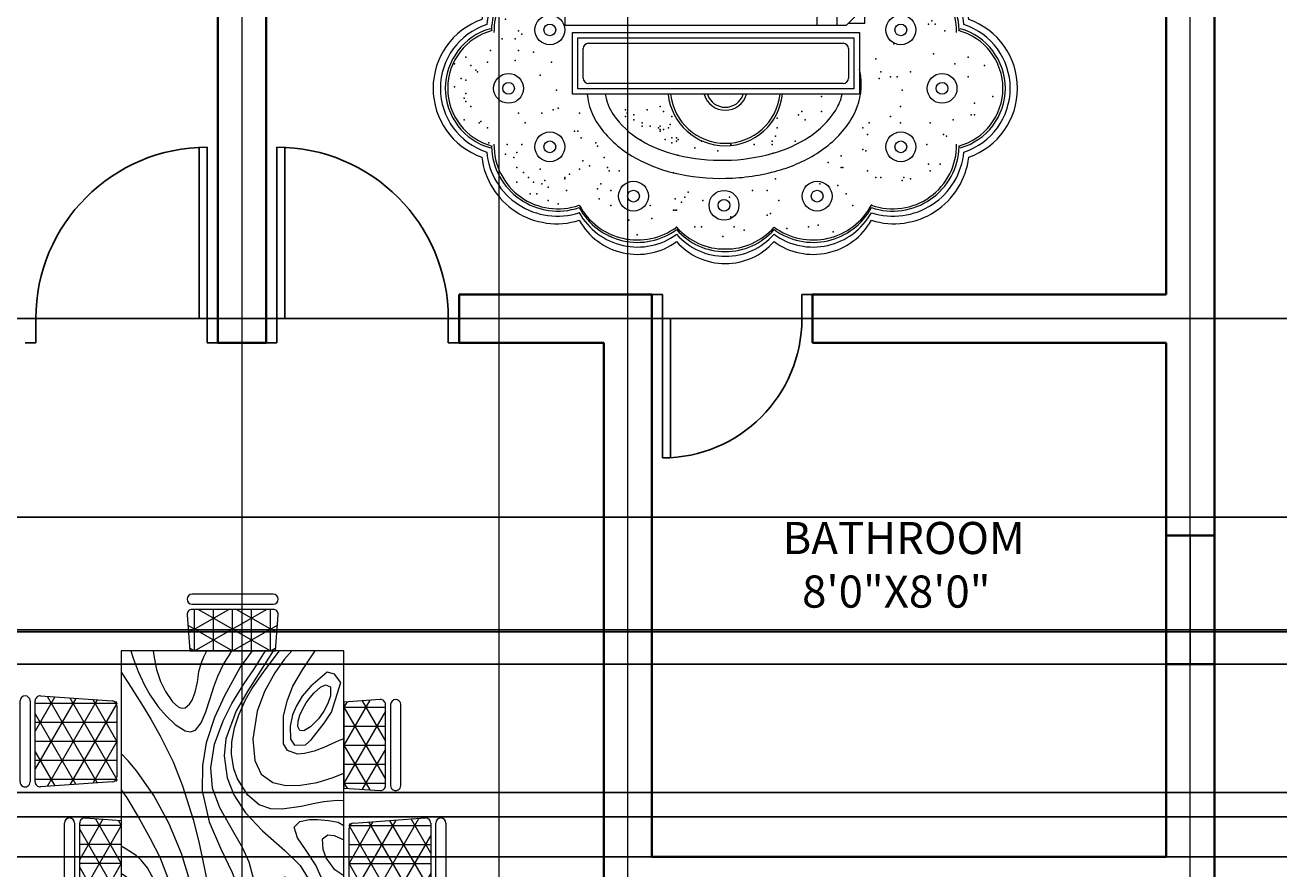
# Model space of a CAD drawing. Units: inches. Extents: x 5716 to 6907, y 12769 to 13594.
# Tile 15 of 17: x 6414 to 6648, y 13192 to 13349. Entities that reach past the tile are written whole.
import ezdxf

# ---------------------------------------------------------------- set-up
doc = ezdxf.new("R2010")
doc.units = ezdxf.units.IN
doc.linetypes.add('ACAD_ISO03W100', pattern=[30, 12, -18])
for name, color, linetype, lineweight in [('A-ANNO-DIMS', 2, 'Continuous', 18), ('A-AREA-IDEN', 7, 'Continuous', 18), ('A-DOOR', 4, 'Continuous', 25), ('A-FLOR-OVHD', 8, 'ACAD_ISO03W100', 18), ('A-FURN', 8, 'Continuous', 18), ('A-GLAZ', 4, 'Continuous', 18), ('A-GRID', 8, 'Continuous', 13), ('A-WALL', 7, 'Continuous', 35)]:
    doc.layers.add(name, color=color, linetype=linetype, lineweight=lineweight)
doc.styles.get("Standard").update_dxf_attribs({"font": 'arial.ttf'})
doc.dimstyles.get("Standard").update_dxf_attribs({"dimtxt": 0.18, "dimasz": 0.18, "dimexe": 0.18, "dimexo": 0.0625, "dimgap": 0.09, "dimtad": 0, "dimtih": 1, "dimtoh": 1, "dimdec": 4, "dimzin": 0, "dimdsep": 46, "dimtxsty": 'Standard', "dimcen": 0.09, "dimadec": 0, "dimazin": 0, "dimtfac": 1, "dimtdec": 4, "dimtofl": 0, "dimtmove": 0, "dimatfit": 3, "dimfxl": 1, "dimtolj": 1, "dimtzin": 0, "dimarcsym": 0})

# ---------------------------------------------------------------- blocks, each defined once
blk = doc.blocks.new('A$C1EC128A1')
for p, q in [((0.1147, 3.56), (3.0187, 3.56)), ((0.1147, 3.555), (0.1147, 3.511)), ((3.0187, 3.555), (3.0187, 3.511)), ((0.1147, 3.511), (3.0187, 3.511)), ((0.2027, 3.511), (0.2027, 3.4616)), ((0.6977, 3.511), (0.6977, 3.016)), ((0.7417, 3.511), (0.7417, 2.972)), ((0.7857, 3.4835), (1.5392, 3.4835)), ((0.7857, 3.4835), (0.7857, 3.126)), ((1.5392, 3.126), (1.5392, 3.4835)), ((1.5942, 3.126), (1.5942, 3.4835)), ((1.5942, 3.4835), (2.3477, 3.4835)), ((2.3477, 3.4835), (2.3477, 3.126)), ((2.3917, 3.511), (2.3917, 3.1535)), ((2.4357, 3.511), (2.4357, 3.016)), ((2.9307, 3.511), (2.9307, 3.016)), ((0.2027, 3.4601), (0.2027, 3.016)), ((0.3741, 3.1815), (0.5297, 3.337)), ((0.3741, 3.337), (0.5297, 3.1815)), ((2.6038, 3.337), (2.7594, 3.1815)), ((2.7594, 3.337), (2.6038, 3.1815)), ((1.5392, 3.1535), (1.5942, 3.1535)), ((2.3477, 3.1535), (2.4027, 3.1535)), ((2.4027, 3.1535), (2.4027, 1.432)), ((0.7307, 2.961), (0.8957, 3.126)), ((0.7857, 3.126), (1.5392, 3.126)), ((0.9507, 3.126), (0.9507, 2.9335)), ((1.0607, 3.126), (1.0607, 2.8235)), ((1.5942, 3.126), (2.3477, 3.126)), ((0.2027, 3.016), (0.6977, 3.016)), ((1.0607, 3.0435), (2.4027, 3.0435)), ((2.9307, 3.016), (2.4357, 3.016)), ((0.7307, 2.961), (0.7307, 1.322)), ((0.7307, 2.9335), (0.9507, 2.9335)), ((0.7307, 2.8235), (1.0607, 2.8235)), ((2.1277, 1.597), (2.4027, 1.597)), ((2.1277, 1.597), (2.1277, 1.322)), ((2.2377, 1.487), (2.2377, 1.322)), ((2.2377, 1.487), (2.4027, 1.487)), ((2.2927, 1.322), (2.4027, 1.432)), ((2.3917, 1.421), (2.3917, 1.333)), ((0.7307, 1.322), (2.2927, 1.322)), ((2.3037, 1.333), (2.3917, 1.333)), ((0.7721, 1.282), (2.3633, 1.282)), ((0.7721, 0.939), (0.7721, 1.282)), ((0.8021, 1.252), (2.3333, 1.252)), ((0.8021, 0.969), (0.8021, 1.252)), ((2.3333, 1.252), (2.3333, 0.969)), ((2.3633, 1.282), (2.3633, 0.939)), ((0.8321, 1.029), (0.8321, 1.192)), ((0.8621, 1.222), (2.2733, 1.222)), ((2.3033, 1.192), (2.3033, 1.029)), ((2.2733, 0.999), (0.8621, 0.999)), ((2.3633, 0.939), (0.7721, 0.939)), ((2.3333, 0.969), (0.8021, 0.969))]:
    blk.add_line(p, q)
for centre, radius in [((0.4519, 3.2593), 0.22), ((2.6816, 3.2593), 0.22), ((0.4519, 3.2593), 0.11), ((2.6816, 3.2593), 0.11), ((0.647, 1.2961), 0.0826), ((0.647, 1.2961), 0.0326), ((2.593, 1.2961), 0.0826), ((2.593, 1.2961), 0.0326), ((0.4183, 0.9718), 0.0826), ((2.8217, 0.9718), 0.0826), ((0.4183, 0.9718), 0.0326), ((2.8217, 0.9718), 0.0326), ((0.647, 0.6475), 0.0826), ((2.593, 0.6475), 0.0826), ((0.647, 0.6475), 0.0326), ((2.593, 0.6475), 0.0326), ((1.1109, 0.3741), 0.0826), ((2.1291, 0.3741), 0.0826), ((1.1109, 0.3741), 0.0326), ((1.6128, 0.3232), 0.0826), ((1.6128, 0.3232), 0.0326), ((2.1291, 0.3741), 0.0326)]:
    blk.add_circle(centre, radius)
for centre, radius, start, end in [((0.6854, 1.3045), 0.4183, 83.78243, 173.25148), ((0.6884, 1.2877), 0.3932, 83.81567, 174.52996), ((2.5546, 1.3045), 0.4183, 6.74852, 111.27952), ((2.5516, 1.2877), 0.3932, 5.47004, 112.24899), ((0.6921, 1.2838), 0.369, 83.99709, 177.99757), ((0.6913, 1.2866), 0.3539, 83.60511, 180.66989), ((2.5479, 1.2838), 0.369, 2.00243, 113.15364), ((2.5487, 1.2866), 0.3539, 359.33011, 114.35507), ((0.4048, 0.972), 0.4048, 109.45268, 180), ((0.4119, 0.972), 0.3714, 108.02557, 180), ((2.8281, 0.972), 0.3714, 0, 71.97443), ((2.8352, 0.972), 0.4048, 0, 70.54732), ((0.411, 0.972), 0.3435, 105.78906, 180), ((0.4122, 0.972), 0.3312, 104.76604, 180), ((2.8278, 0.972), 0.3312, 0, 75.23396), ((2.829, 0.972), 0.3435, 0, 74.21094), ((0.8621, 1.192), 0.03, 90, 180), ((2.2733, 1.192), 0.03, 0, 90), ((2.0084, 0.9935), 0.365, 1.17824, 13.48124), ((0.8621, 1.029), 0.03, 180, 270), ((2.2733, 1.029), 0.03, 270, 0), ((2.0084, 0.9935), 0.365, 327.62391, 1.17824), ((0.4048, 0.972), 0.4048, 180, 250.54732), ((0.4119, 0.972), 0.3714, 180, 251.97443), ((0.411, 0.972), 0.3435, 180, 254.21094), ((0.4122, 0.972), 0.3312, 180, 255.23396), ((1.2169, 0.9773), 0.365, 186.01972, 214.73257), ((1.2169, 0.9773), 0.265, 188.30546, 214.73257), ((1.62, 0.972), 0.3185, 185.95071, 354.04929), ((1.62, 0.972), 0.305, 186.21512, 353.78488), ((1.62, 0.972), 0.1215, 195.7695, 344.2305), ((1.62, 0.972), 0.105, 198.32909, 341.67091), ((2.0084, 0.9935), 0.265, 327.62391, 348.11864), ((2.8278, 0.972), 0.3312, 284.76604, 0), ((2.829, 0.972), 0.3435, 285.78906, 0), ((2.8281, 0.972), 0.3714, 288.02557, 0), ((2.8352, 0.972), 0.4048, 289.45268, 0), ((1.8167, 1.1151), 0.492, 303.16388, 327.62391), ((1.4035, 1.1066), 0.592, 214.73257, 239.1926), ((1.4035, 1.1066), 0.492, 214.73257, 239.1926), ((1.8167, 1.1151), 0.592, 303.16388, 327.62391), ((1.6878, 1.3123), 0.7275, 285.68186, 303.16388), ((0.6921, 0.6602), 0.369, 182.00243, 288.62304), ((0.6913, 0.6574), 0.3539, 179.33011, 289.59453), ((1.5241, 1.3089), 0.7275, 239.1926, 256.67462), ((2.5487, 0.6574), 0.3539, 250.40547, 0.66989), ((2.5479, 0.6602), 0.369, 251.37696, 357.99757), ((0.6854, 0.6395), 0.4183, 186.74852, 287.32326), ((0.6884, 0.6563), 0.3932, 185.47004, 288.01752), ((1.5241, 1.3089), 0.8275, 239.1926, 256.67462), ((1.5995, 1.627), 1.0544, 256.67462, 271.17824), ((1.5995, 1.627), 1.0544, 271.17824, 285.68186), ((1.6878, 1.3123), 0.8275, 285.68186, 303.16388), ((2.5516, 0.6563), 0.3932, 251.98248, 354.52996), ((2.5546, 0.6395), 0.4183, 252.67674, 353.25148), ((1.5995, 1.627), 1.1544, 256.67462, 271.17824), ((1.5995, 1.627), 1.1544, 271.17824, 285.68186), ((1.1328, 0.4977), 0.3665, 208.29135, 306.34788), ((1.1328, 0.4842), 0.3665, 208.29135, 306.34788), ((1.133, 0.4609), 0.369, 208.93019, 306.02618), ((2.1072, 0.4977), 0.3665, 233.65212, 331.70865), ((2.1072, 0.4842), 0.3665, 233.65212, 331.70865), ((2.107, 0.4609), 0.369, 233.97382, 331.06981), ((1.1324, 0.4204), 0.3694, 209.22014, 306.07902), ((2.1076, 0.4204), 0.3694, 233.92098, 330.77986), ((1.6145, 0.4295), 0.3486, 220.6393, 270.90521), ((1.6145, 0.416), 0.3486, 220.6393, 270.90521), ((1.62, 0.4004), 0.3599, 221.38778, 270), ((1.6255, 0.4295), 0.3486, 269.09479, 319.3607), ((1.6255, 0.416), 0.3486, 269.09479, 319.3607), ((1.62, 0.4004), 0.3599, 270, 318.61222), ((1.62, 0.36), 0.36, 221.41854, 270), ((1.62, 0.36), 0.36, 270, 318.58146)]:
    blk.add_arc(centre, radius, start, end)
for p in [(0.5654, 1.5652), (0.6657, 1.5561), (2.4819, 1.5378), (2.5184, 1.5744), (2.5366, 1.5378), (2.6097, 1.5378), (2.71, 1.5561), (0.4376, 1.5104), (0.465, 1.4739), (0.5471, 1.5013), (0.5471, 1.4922), (0.6475, 1.5013), (2.6735, 1.4739), (0.4285, 1.4282), (0.4285, 1.3917), (0.5562, 1.3917), (0.5927, 1.3917), (0.6566, 1.41), (2.6005, 1.4191), (2.6735, 1.4556), (2.7648, 1.4465), (2.8013, 1.4191), (0.4011, 1.3552), (0.4285, 1.3734), (2.3917, 1.333), (2.7465, 1.3278), (2.7648, 1.346), (2.7831, 1.3278), (0.4741, 1.2912), (0.4923, 1.273), (2.8378, 1.2912), (0.3828, 1.2456), (0.4558, 1.2456), (2.5549, 1.2182), (0.1821, 1.1451), (0.3007, 1.1177), (0.3189, 1.1816), (0.4558, 1.1268), (0.4741, 1.1816), (0.5562, 1.1725), (0.6566, 1.1177), (2.4545, 1.1359), (2.7739, 1.1634), (2.9656, 1.1451), (0.1182, 1.1085), (0.2094, 1.0994), (0.2368, 1.072), (0.2459, 1.0629), (0.5927, 1.0446), (2.4819, 1.0629), (2.6462, 1.0629), (2.8926, 1.1085), (3.0568, 1.0994), (0.1182, 0.9807), (0.1547, 1.0263), (0.1821, 1.0172), (2.4728, 1.0263), (2.5366, 1.0355), (2.5731, 1.0355), (2.9656, 1.0355), (0.1729, 0.9167), (0.1821, 0.9441), (0.684, 0.9624), (1.3032, 0.939), (1.3168, 0.939), (2.1533, 0.9259), (2.6005, 0.9624), (3.1025, 0.9259), (0.1821, 0.8985), (0.2094, 0.8711), (0.4741, 0.8345), (0.6019, 0.8345), (0.6657, 0.8528), (0.6931, 0.8619), (0.8118, 0.8345), (1.0673, 0.8528), (1.0764, 0.8345), (1.1859, 0.8528), (1.259, 0.8711), (1.2772, 0.8437), (2.0438, 0.8437), (2.0438, 0.8437), (2.1533, 0.8437), (2.5914, 0.8711), (3.0021, 0.8893), (0.1729, 0.798), (0.2551, 0.7797), (0.2642, 0.7889), (0.5106, 0.7797), (0.9992, 0.8263), (1.0673, 0.8163), (1.1129, 0.8254), (1.1129, 0.798), (1.1586, 0.7797), (1.3137, 0.7706), (1.3228, 0.8163), (1.9069, 0.8071), (2.0256, 0.8254), (2.0621, 0.798), (2.418, 0.7797), (2.5366, 0.8163), (2.5914, 0.7797), (2.7557, 0.7797), (2.8834, 0.798), (2.9838, 0.8254), (3.0021, 0.8254), (0.3007, 0.7523), (0.7844, 0.7341), (0.8026, 0.7341), (0.8209, 0.6975), (1.1586, 0.7615), (1.2042, 0.7615), (1.2498, 0.7523), (1.259, 0.7615), (1.259, 0.7432), (1.259, 0.7341), (1.2772, 0.7432), (1.3046, 0.7523), (1.3228, 0.6975), (1.3502, 0.6975), (1.8978, 0.7067), (1.9069, 0.7523), (2.0858, 0.7033), (2.3815, 0.7523), (2.4089, 0.7158), (2.8287, 0.7158), (2.8469, 0.7067), (0.3098, 0.6701), (0.4102, 0.661), (0.4923, 0.661), (0.903, 0.6701), (0.9122, 0.6519), (1.1515, 0.684), (1.1515, 0.684), (1.1515, 0.684), (1.2863, 0.6884), (1.3228, 0.6701), (1.3502, 0.6793), (1.3593, 0.6884), (1.4506, 0.6427), (1.4871, 0.6793), (1.6514, 0.661), (1.6514, 0.661), (1.7792, 0.661), (1.8795, 0.6793), (1.8795, 0.661), (2.0073, 0.6793), (2.3815, 0.6336), (2.7374, 0.661), (0.4011, 0.6062), (0.4467, 0.5879), (0.465, 0.6153), (0.83, 0.5696), (0.9487, 0.5879), (1.3564, 0.601), (1.5784, 0.6245), (1.8845, 0.6118), (2.1898, 0.5605), (2.2629, 0.597), (2.3997, 0.6245), (0.465, 0.5331), (0.5015, 0.5057), (0.5927, 0.524), (0.757, 0.4966), (0.8118, 0.524), (0.8665, 0.5422), (0.9669, 0.5331), (0.976, 0.5148), (1.0308, 0.5148), (1.3334, 0.5037), (2.2629, 0.5331), (2.272, 0.5331), (2.4089, 0.5148), (2.7465, 0.5514), (2.7557, 0.5148), (2.8104, 0.5514), (0.465, 0.4509), (0.5289, 0.4783), (0.5562, 0.4509), (0.6019, 0.4418), (0.6201, 0.46), (0.6384, 0.4235), (0.7296, 0.4783), (0.7296, 0.4692), (0.9304, 0.4418), (1.8978, 0.4692), (2.1442, 0.4418), (2.2446, 0.4326), (2.4545, 0.4783), (2.4819, 0.4783), (2.6005, 0.46), (2.6097, 0.4783), (2.6462, 0.4692), (0.538, 0.387), (0.5745, 0.387), (0.6384, 0.3504), (0.7388, 0.4052), (0.7388, 0.4052), (0.9122, 0.4144), (0.9213, 0.3596), (0.9852, 0.4052), (1.3411, 0.3596), (1.3959, 0.3687), (1.4141, 0.3961), (1.4962, 0.3504), (1.6423, 0.3687), (1.77, 0.4052), (1.8522, 0.4052), (1.9161, 0.3504), (2.2902, 0.387), (0.6931, 0.3322), (0.81, 0.2824), (0.9852, 0.323), (1.2042, 0.323), (1.332, 0.2956), (1.3411, 0.2956), (1.3502, 0.2956), (1.3776, 0.3413), (2.3267, 0.323), (2.43, 0.324), (1.0856, 0.2408), (1.2133, 0.25), (1.6514, 0.2591), (1.8522, 0.2682), (1.8704, 0.2774), (2.1351, 0.2134), (0.9852, 0.1495), (1.1312, 0.1586), (1.35, 0.2025), (1.4506, 0.2043), (1.4871, 0.2043), (1.6058, 0.1495), (1.6696, 0.2043), (1.7244, 0.186), (1.9617, 0.1952), (2.0803, 0.2043), (2.2172, 0.1769)]:
    blk.add_point(p)
blk = doc.blocks.new('A$C405465A0')
for p, q in [((1.1305, 2.1034), (1.5301, 2.1034)), ((1.5301, 2.0534), (1.1305, 2.0534)), ((1.1304, 1.6481), (1.1055, 2.0017)), ((1.279, 2.0284), (1.1105, 1.9312)), ((1.4665, 2.0284), (1.1178, 1.8271)), ((1.1305, 2.0284), (1.5301, 2.0284)), ((1.1428, 1.625), (1.1428, 2.0284)), ((1.5427, 1.8271), (1.1941, 2.0284)), ((1.2365, 1.625), (1.2365, 2.0284)), ((1.3303, 1.625), (1.3303, 2.0284)), ((1.5501, 1.9312), (1.3816, 2.0284)), ((1.424, 1.625), (1.424, 2.0284)), ((1.5178, 1.625), (1.5178, 2.0284)), ((1.555, 2.0017), (1.5301, 1.6481)), ((1.5354, 1.7231), (1.1078, 1.97)), ((1.5528, 1.97), (1.1252, 1.7231)), ((0.9452, 1.8803), (0.5455, 1.8803)), ((2.1342, 1.8803), (1.7345, 1.8803)), ((0.5268, 1.6904), (0.7259, 1.8053)), ((0.5455, 1.8303), (0.9452, 1.8303)), ((0.9452, 1.8053), (0.5455, 1.8053)), ((0.5578, 1.6), (0.5578, 1.8053)), ((0.5578, 1.6), (0.9134, 1.8053)), ((0.5773, 1.8053), (0.9328, 1.6)), ((0.6516, 1.6), (0.6516, 1.8053)), ((0.7453, 1.6), (0.7453, 1.8053)), ((0.7648, 1.8053), (0.9639, 1.6904)), ((0.8391, 1.6), (0.8391, 1.8053)), ((0.9328, 1.6), (0.9328, 1.8053)), ((1.5178, 1.625), (1.1157, 1.8572)), ((1.5449, 1.8572), (1.1428, 1.625)), ((1.7158, 1.6904), (1.9149, 1.8053)), ((1.7345, 1.8303), (2.1342, 1.8303)), ((2.1342, 1.8053), (1.7345, 1.8053)), ((1.7468, 1.6), (1.7468, 1.8053)), ((1.7468, 1.6), (2.1024, 1.8053)), ((1.7663, 1.8053), (2.1218, 1.6)), ((1.8406, 1.6), (1.8406, 1.8053)), ((1.9343, 1.6), (1.9343, 1.8053)), ((1.9538, 1.8053), (2.1529, 1.6904)), ((2.0281, 1.6), (2.0281, 1.8053)), ((2.1218, 1.6), (2.1218, 1.8053)), ((0.5206, 1.7786), (0.5332, 1.6)), ((0.9575, 1.6), (0.9701, 1.7786)), ((1.3303, 1.625), (1.1237, 1.7443)), ((1.5369, 1.7443), (1.3303, 1.625)), ((1.7096, 1.7786), (1.7222, 1.6)), ((2.1465, 1.6), (2.1591, 1.7786)), ((0.5242, 1.7277), (0.7453, 1.6)), ((0.7453, 1.6), (0.9665, 1.7277)), ((1.7132, 1.7277), (1.9343, 1.6)), ((1.9343, 1.6), (2.1555, 1.7277)), ((0.5321, 1.6149), (0.5578, 1.6)), ((0.9328, 1.6), (0.9586, 1.6149)), ((1.1428, 1.625), (1.1316, 1.6315)), ((1.5052, 1.625), (1.1554, 1.625)), ((1.529, 1.6315), (1.5178, 1.625)), ((1.7211, 1.6149), (1.7468, 1.6)), ((2.1218, 1.6), (2.1476, 1.6149)), ((2.3803, 1.6), (0.2803, 1.6)), ((0.2803, 1.6), (0.2803, 0.5)), ((0.3956, 1.553), (0.3856, 1.5163)), ((0.4356, 1.5842), (0.3956, 1.553)), ((0.5827, 1.5379), (0.4356, 1.5842)), ((0.5332, 1.6), (0.9575, 1.6)), ((0.7152, 1.6), (0.7236, 1.5766)), ((0.7236, 1.5766), (0.7578, 1.4998)), ((0.9055, 1.5469), (0.8836, 1.6)), ((1.0212, 1.6), (1.0194, 1.5656)), ((1.0194, 1.5656), (1.026, 1.5003)), ((1.1178, 1.5243), (1.1269, 1.5706)), ((1.1269, 1.5706), (1.1432, 1.6)), ((1.1887, 1.5196), (1.1922, 1.5507)), ((1.1922, 1.5507), (1.214, 1.6)), ((1.3616, 1.5541), (1.3027, 1.5125)), ((1.3907, 1.6), (1.3616, 1.5541)), ((1.7222, 1.6), (2.1465, 1.6)), ((1.9093, 1.5754), (1.8386, 1.5427)), ((1.9386, 1.6), (1.9093, 1.5754)), ((1.9962, 1.5248), (2.1086, 1.5664)), ((2.1086, 1.5664), (2.17, 1.6)), ((2.3153, 1.558), (2.1962, 1.4994)), ((2.3803, 1.5967), (2.3153, 1.558)), ((2.3803, 0.5), (2.3803, 1.6)), ((0.3856, 1.5163), (0.4538, 1.4363)), ((0.4482, 1.5094), (0.4582, 1.5336)), ((0.4595, 1.4847), (0.4482, 1.5094)), ((0.4582, 1.5336), (0.5016, 1.5339)), ((0.5016, 1.5339), (0.54, 1.5204)), ((0.54, 1.5204), (0.5786, 1.5)), ((0.5786, 1.5), (0.6151, 1.4744)), ((0.6365, 1.5019), (0.5827, 1.5379)), ((0.7193, 1.4377), (0.6365, 1.5019)), ((0.7578, 1.4998), (0.7752, 1.4525)), ((0.9296, 1.4669), (0.9055, 1.5469)), ((1.026, 1.5003), (1.0343, 1.4559)), ((1.1128, 1.4699), (1.1178, 1.5243)), ((1.2089, 1.4946), (1.1887, 1.5196)), ((1.2618, 1.4976), (1.2089, 1.4946)), ((1.3027, 1.5125), (1.2618, 1.4976)), ((1.446, 1.5079), (1.3392, 1.4609)), ((1.5543, 1.5261), (1.446, 1.5079)), ((1.6627, 1.5271), (1.5543, 1.5261)), ((1.7679, 1.5301), (1.6627, 1.5271)), ((1.717, 1.474), (1.8488, 1.4892)), ((1.8386, 1.5427), (1.7679, 1.5301)), ((1.8488, 1.4892), (1.9962, 1.5248)), ((2.1962, 1.4994), (2.0887, 1.4564)), ((2.215, 1.4381), (2.3447, 1.5068)), ((2.3447, 1.5068), (2.3803, 1.5269)), ((0.3744, 1.3943), (0.2803, 1.458)), ((0.4538, 1.4363), (0.5034, 1.394)), ((0.4876, 1.4521), (0.4595, 1.4847)), ((0.5099, 1.4328), (0.4876, 1.4521)), ((0.5366, 1.4137), (0.5099, 1.4328)), ((0.6151, 1.4744), (0.6557, 1.4351)), ((0.6557, 1.4351), (0.6746, 1.4025)), ((0.7442, 1.4091), (0.7193, 1.4377)), ((0.7752, 1.4525), (0.7871, 1.4053)), ((0.9436, 1.385), (0.9296, 1.4669)), ((1.0343, 1.4559), (1.0488, 1.3883)), ((1.1133, 1.4295), (1.1128, 1.4699)), ((1.1222, 1.3821), (1.1133, 1.4295)), ((1.3392, 1.4609), (1.2655, 1.4131)), ((1.3398, 1.3841), (1.4396, 1.445)), ((1.4396, 1.445), (1.5179, 1.4625)), ((1.5179, 1.4625), (1.717, 1.474)), ((1.9879, 1.4268), (1.8502, 1.4019)), ((2.0887, 1.4564), (1.9879, 1.4268)), ((2.1089, 1.3912), (2.215, 1.4381)), ((0.4543, 1.3479), (0.3744, 1.3943)), ((0.5034, 1.394), (0.551, 1.3648)), ((0.5694, 1.3947), (0.5366, 1.4137)), ((0.551, 1.3648), (0.5952, 1.3458)), ((0.597, 1.3823), (0.5694, 1.3947)), ((0.6281, 1.3731), (0.597, 1.3823)), ((0.654, 1.3714), (0.6281, 1.3731)), ((0.674, 1.3825), (0.654, 1.3714)), ((0.6746, 1.4025), (0.674, 1.3825)), ((0.746, 1.3555), (0.7442, 1.4091)), ((0.7898, 1.3706), (0.7722, 1.3216)), ((0.7871, 1.4053), (0.7898, 1.3706)), ((0.9447, 1.3133), (0.9436, 1.385)), ((1.0488, 1.3883), (1.0626, 1.2943)), ((1.1508, 1.3537), (1.1222, 1.3821)), ((1.2034, 1.3712), (1.1508, 1.3537)), ((1.2655, 1.4131), (1.2034, 1.3712)), ((1.2659, 1.3078), (1.3398, 1.3841)), ((1.4616, 1.3726), (1.4211, 1.3426)), ((1.5407, 1.3902), (1.4616, 1.3726)), ((1.6315, 1.3907), (1.5407, 1.3902)), ((1.7291, 1.3922), (1.6315, 1.3907)), ((1.8502, 1.4019), (1.7291, 1.3922)), ((1.8869, 1.3472), (1.9689, 1.3731)), ((1.9689, 1.3731), (2.0551, 1.3789)), ((2.0551, 1.3789), (2.1089, 1.3912)), ((2.1327, 1.3477), (2.1998, 1.3905)), ((2.1998, 1.3905), (2.271, 1.4021)), ((2.271, 1.4021), (2.3264, 1.3943)), ((2.3264, 1.3943), (2.3803, 1.3943)), ((0.2803, 1.3424), (0.3226, 1.3046)), ((0.3226, 1.3046), (0.3891, 1.2586)), ((0.523, 1.3203), (0.4543, 1.3479)), ((0.6007, 1.301), (0.523, 1.3203)), ((0.5952, 1.3458), (0.6524, 1.335)), ((0.6623, 1.3018), (0.6007, 1.301)), ((0.6524, 1.335), (0.7159, 1.3352)), ((0.7385, 1.3018), (0.6623, 1.3018)), ((0.7159, 1.3352), (0.746, 1.3555)), ((0.7722, 1.3216), (0.7385, 1.3018)), ((0.9305, 1.2479), (0.9447, 1.3133)), ((1.1689, 1.1968), (1.2659, 1.3078)), ((1.4211, 1.3426), (1.398, 1.3071)), ((1.398, 1.3071), (1.412, 1.2681)), ((1.8267, 1.2783), (1.8309, 1.3257)), ((1.8309, 1.3257), (1.8869, 1.3472)), ((2.1112, 1.3052), (2.1327, 1.3477)), ((2.1264, 1.2714), (2.1112, 1.3052)), ((2.2336, 1.2914), (2.2346, 1.3391)), ((2.2346, 1.3391), (2.2726, 1.3593)), ((2.2726, 1.3593), (2.339, 1.3581)), ((2.339, 1.3581), (2.3803, 1.3581)), ((0, 1.2499), (0, 0.8502)), ((0.05, 0.8502), (0.05, 1.2499)), ((0.075, 1.0695), (0.19, 1.2686)), ((0.075, 1.2499), (0.075, 0.8502)), ((0.2803, 1.2622), (0.1018, 1.2748)), ((0.2803, 1.05), (0.1526, 1.2712)), ((0.2803, 1.2375), (0.2654, 1.2633)), ((0.3797, 1.2052), (0.2803, 1.2816)), ((0.2803, 0.8379), (0.2803, 1.2622)), ((0.2803, 1.2498), (0.478, 1.1251)), ((0.3891, 1.2586), (0.4808, 1.2074)), ((0.8894, 1.1911), (0.9305, 1.2479)), ((1.06, 1.2384), (1.0402, 1.1815)), ((1.0626, 1.2943), (1.06, 1.2384)), ((1.412, 1.2681), (1.4535, 1.2416)), ((1.4535, 1.2416), (1.5203, 1.2085)), ((1.8814, 1.2462), (1.8267, 1.2783)), ((1.9819, 1.2225), (1.8814, 1.2462)), ((2.171, 1.2386), (2.1264, 1.2714)), ((2.2593, 1.2028), (2.171, 1.2386)), ((2.2746, 1.2504), (2.2336, 1.2914)), ((2.3417, 1.2285), (2.2746, 1.2504)), ((2.3803, 1.2622), (2.5588, 1.2748)), ((2.3803, 1.05), (2.508, 1.2712)), ((2.3803, 1.2375), (2.3951, 1.2633)), ((2.3803, 0.8379), (2.3803, 1.2622)), ((2.5856, 1.0695), (2.4706, 1.2686)), ((2.5856, 1.2499), (2.5856, 0.8502)), ((2.6106, 0.8502), (2.6106, 1.2499)), ((2.6606, 1.2499), (2.6606, 0.8502)), ((0.2803, 1.2375), (0.075, 1.2375)), ((0.075, 0.882), (0.2803, 1.2375)), ((0.2803, 0.8625), (0.075, 1.2181)), ((0.3728, 1.1548), (0.2803, 1.2123)), ((0.4682, 1.1454), (0.3797, 1.2052)), ((0.4808, 1.2074), (0.5771, 1.1712)), ((0.8213, 1.159), (0.8894, 1.1911)), ((1.0402, 1.1815), (0.9932, 1.1252)), ((1.0809, 1.1136), (1.1689, 1.1968)), ((1.5203, 1.2085), (1.5912, 1.2143)), ((1.5912, 1.2143), (1.7027, 1.2151)), ((1.7027, 1.2151), (1.8282, 1.1987)), ((1.8282, 1.1987), (1.9236, 1.1792)), ((1.9236, 1.1792), (2.049, 1.1552)), ((2.1048, 1.2108), (1.9819, 1.2225)), ((2.1888, 1.194), (2.1048, 1.2108)), ((2.2653, 1.1704), (2.1888, 1.194)), ((2.3339, 1.1841), (2.2593, 1.2028)), ((2.3803, 1.1754), (2.3339, 1.1841)), ((2.3803, 1.226), (2.3417, 1.2285)), ((2.3803, 1.2375), (2.5856, 1.2375)), ((2.5856, 0.882), (2.3803, 1.2375)), ((2.3803, 0.8625), (2.5856, 1.2181)), ((0.2803, 1.1438), (0.075, 1.1438)), ((0.2803, 1.1471), (0.3609, 1.0879)), ((0.4405, 1.1078), (0.3728, 1.1548)), ((0.5225, 1.114), (0.4682, 1.1454)), ((0.478, 1.1251), (0.576, 1.067)), ((0.5771, 1.1712), (0.7161, 1.1491)), ((0.7161, 1.1491), (0.8213, 1.159)), ((0.9932, 1.1252), (0.9121, 1.0739)), ((1.3237, 1.1316), (1.2549, 1.1012)), ((1.4537, 1.1662), (1.3237, 1.1316)), ((1.6097, 1.1755), (1.4537, 1.1662)), ((1.757, 1.1624), (1.6097, 1.1755)), ((1.9184, 1.131), (1.757, 1.1624)), ((2.0769, 1.0887), (1.9184, 1.131)), ((2.049, 1.1552), (2.1515, 1.1303)), ((2.1515, 1.1303), (2.2486, 1.0908)), ((2.3396, 1.1432), (2.2653, 1.1704)), ((2.3803, 1.126), (2.3396, 1.1432)), ((2.3803, 1.1438), (2.5856, 1.1438)), ((0.3609, 1.0879), (0.5015, 1.0099)), ((0.5402, 1.0464), (0.4405, 1.1078)), ((0.5954, 1.0801), (0.5225, 1.114)), ((0.576, 1.067), (0.7146, 1.0163)), ((0.6603, 1.0585), (0.5954, 1.0801)), ((0.7308, 1.0454), (0.6603, 1.0585)), ((0.863, 1.056), (0.7897, 1.0439)), ((0.9121, 1.0739), (0.863, 1.056)), ((0.9069, 1.0237), (0.9908, 1.0561)), ((0.9908, 1.0561), (1.0809, 1.1136)), ((1.2549, 1.1012), (1.1432, 1.0368)), ((1.3755, 1.0479), (1.4887, 1.0901)), ((1.4887, 1.0901), (1.6473, 1.1088)), ((1.6473, 1.1088), (1.7544, 1.0961)), ((1.7544, 1.0961), (1.9207, 1.0564)), ((1.9207, 1.0564), (2.1244, 0.9922)), ((2.2686, 1.0282), (2.0769, 1.0887)), ((2.2486, 1.0908), (2.3803, 1.048)), ((0.2803, 1.05), (0.075, 1.05)), ((0.19, 0.8315), (0.075, 1.0306)), ((0.1526, 0.8289), (0.2803, 1.05)), ((0.3078, 1.029), (0.2803, 1.0458)), ((0.346, 1.0052), (0.3078, 1.029)), ((0.4051, 0.9771), (0.346, 1.0052)), ((0.5015, 1.0099), (0.6086, 0.961)), ((0.6261, 1.0028), (0.5402, 1.0464)), ((0.7415, 0.9604), (0.6261, 1.0028)), ((0.7146, 1.0163), (0.7979, 1.0084)), ((0.7897, 1.0439), (0.7308, 1.0454)), ((0.7979, 1.0084), (0.9069, 1.0237)), ((1.1432, 1.0368), (1.0559, 0.9876)), ((1.1244, 0.9348), (1.2543, 0.9907)), ((1.2543, 0.9907), (1.3755, 1.0479)), ((2.1244, 0.9922), (2.2495, 0.9522)), ((2.3803, 0.9983), (2.2686, 1.0282)), ((2.3803, 1.05), (2.5856, 1.05)), ((2.508, 0.8289), (2.3803, 1.05)), ((2.4706, 0.8315), (2.5856, 1.0306)), ((0.2803, 0.9563), (0.075, 0.9563)), ((0.4579, 0.9575), (0.4051, 0.9771)), ((0.5195, 0.9378), (0.4579, 0.9575)), ((0.5818, 0.918), (0.5195, 0.9378)), ((0.6086, 0.961), (0.7339, 0.9201)), ((0.8579, 0.9417), (0.7415, 0.9604)), ((0.958, 0.9508), (0.8579, 0.9417)), ((1.0559, 0.9876), (0.958, 0.9508)), ((0.9714, 0.9002), (1.1244, 0.9348)), ((1.4378, 0.9282), (1.5224, 0.9439)), ((1.5224, 0.9439), (1.6187, 0.9581)), ((1.6187, 0.9581), (1.7607, 0.9676)), ((1.7607, 0.9676), (1.9339, 0.9563)), ((1.9339, 0.9563), (2.0478, 0.9301)), ((2.0478, 0.9301), (2.1209, 0.9013)), ((2.2495, 0.9522), (2.3803, 0.9025)), ((2.3803, 0.9563), (2.5856, 0.9563)), ((0.309, 0.9074), (0.2803, 0.9224)), ((0.342, 0.8943), (0.309, 0.9074)), ((0.3823, 0.8837), (0.342, 0.8943)), ((0.4349, 0.876), (0.3823, 0.8837)), ((0.4843, 0.8652), (0.4349, 0.876)), ((0.6352, 0.8954), (0.5818, 0.918)), ((0.6712, 0.8671), (0.6352, 0.8954)), ((0.6805, 0.8424), (0.6712, 0.8671)), ((0.7339, 0.9201), (0.8463, 0.9008)), ((0.8463, 0.9008), (0.9714, 0.9002)), ((1.1125, 0.8545), (1.224, 0.8829)), ((1.224, 0.8829), (1.301, 0.9003)), ((1.301, 0.9003), (1.4378, 0.9282)), ((1.6341, 0.8806), (1.5313, 0.864)), ((1.7415, 0.8904), (1.6341, 0.8806)), ((1.8296, 0.8853), (1.7415, 0.8904)), ((1.9317, 0.8609), (1.8296, 0.8853)), ((2.1209, 0.9013), (2.214, 0.8459)), ((0.2803, 0.8625), (0.075, 0.8625)), ((0.1018, 0.8253), (0.2803, 0.8379)), ((0.2654, 0.8368), (0.2803, 0.8625)), ((0.5229, 0.85), (0.4843, 0.8652)), ((0.5441, 0.8372), (0.5229, 0.85)), ((0.5622, 0.8164), (0.5441, 0.8372)), ((0.5634, 0.7968), (0.5622, 0.8164)), ((0.6434, 0.7666), (0.675, 0.8159)), ((0.675, 0.8159), (0.6805, 0.8424)), ((0.9468, 0.8025), (1.1125, 0.8545)), ((1.3995, 0.834), (1.2818, 0.7979)), ((1.5313, 0.864), (1.3995, 0.834)), ((2.0406, 0.8138), (1.9317, 0.8609)), ((2.1229, 0.7618), (2.0406, 0.8138)), ((2.214, 0.8459), (2.297, 0.7736)), ((2.3803, 0.8625), (2.5856, 0.8625)), ((2.3951, 0.8368), (2.3803, 0.8625)), ((2.5588, 0.8253), (2.3803, 0.8379)), ((0.4801, 0.7185), (0.5313, 0.7537)), ((0.5313, 0.7537), (0.5562, 0.7809)), ((0.5562, 0.7809), (0.5634, 0.7968)), ((0.603, 0.7231), (0.6434, 0.7666)), ((0.6995, 0.6921), (0.8288, 0.7556)), ((0.8288, 0.7556), (0.9468, 0.8025)), ((1.2818, 0.7979), (1.131, 0.7357)), ((1.2995, 0.6899), (1.4547, 0.7504)), ((1.4547, 0.7504), (1.6229, 0.7863)), ((1.6229, 0.7863), (1.7436, 0.7907)), ((1.7436, 0.7907), (1.8858, 0.7711)), ((1.8858, 0.7711), (1.9957, 0.7333)), ((2.1698, 0.724), (2.1229, 0.7618)), ((2.297, 0.7736), (2.3432, 0.7176)), ((0.3723, 0.6742), (0.4317, 0.6944)), ((0.4317, 0.6944), (0.4801, 0.7185)), ((0.499, 0.6426), (0.5568, 0.6828)), ((0.5568, 0.6828), (0.603, 0.7231)), ((0.6181, 0.6464), (0.6995, 0.6921)), ((1.131, 0.7357), (0.9946, 0.6604)), ((1.2062, 0.6433), (1.2995, 0.6899)), ((1.4772, 0.6838), (1.4124, 0.6631)), ((1.554, 0.696), (1.4772, 0.6838)), ((1.6333, 0.6993), (1.554, 0.696)), ((1.7153, 0.696), (1.6333, 0.6993)), ((1.7865, 0.6892), (1.7153, 0.696)), ((1.8794, 0.6748), (1.7865, 0.6892)), ((1.9957, 0.7333), (2.0772, 0.6873)), ((2.0772, 0.6873), (2.1261, 0.6491)), ((2.2541, 0.6328), (2.1698, 0.724)), ((2.3432, 0.7176), (2.3803, 0.6555)), ((0.2803, 0.6573), (0.312, 0.6622)), ((0.312, 0.6622), (0.3723, 0.6742)), ((0.4497, 0.615), (0.499, 0.6426)), ((0.5546, 0.6082), (0.6181, 0.6464)), ((0.9946, 0.6604), (0.8746, 0.5766)), ((1.1078, 0.5882), (1.2062, 0.6433)), ((1.3518, 0.6302), (1.3133, 0.5983)), ((1.4124, 0.6631), (1.3518, 0.6302)), ((1.4712, 0.6079), (1.5115, 0.6388)), ((1.5115, 0.6388), (1.5744, 0.6543)), ((1.5188, 0.6159), (1.6031, 0.6361)), ((1.5744, 0.6543), (1.6677, 0.668)), ((1.6031, 0.6361), (1.6918, 0.6436)), ((1.641, 0.6183), (1.6861, 0.6235)), ((1.6677, 0.668), (1.7434, 0.6684)), ((1.6861, 0.6235), (1.7353, 0.624)), ((1.6918, 0.6436), (1.8075, 0.6404)), ((1.7353, 0.624), (1.7765, 0.6204)), ((1.7434, 0.6684), (1.8417, 0.6617)), ((1.7765, 0.6204), (1.811, 0.6136)), ((1.8075, 0.6404), (1.8682, 0.6312)), ((1.8417, 0.6617), (1.8785, 0.6547)), ((1.8682, 0.6312), (1.909, 0.622)), ((1.8785, 0.6547), (1.9243, 0.6434)), ((1.9674, 0.6548), (1.8794, 0.6748)), ((1.909, 0.622), (1.9497, 0.5991)), ((1.9243, 0.6434), (1.9761, 0.6102)), ((2.0494, 0.621), (1.9674, 0.6548)), ((2.1071, 0.5697), (2.0494, 0.621)), ((2.1261, 0.6491), (2.1688, 0.6067)), ((2.3022, 0.5551), (2.2541, 0.6328)), ((0.2803, 0.5477), (0.3159, 0.5583)), ((0.3159, 0.5583), (0.3813, 0.5837)), ((0.3813, 0.5837), (0.4497, 0.615)), ((0.4385, 0.5349), (0.5546, 0.6082)), ((0.8746, 0.5766), (0.8225, 0.5348)), ((1.0064, 0.5273), (1.1078, 0.5882)), ((1.2908, 0.5736), (1.2556, 0.52)), ((1.3133, 0.5983), (1.2908, 0.5736)), ((1.3959, 0.5264), (1.4712, 0.6079)), ((1.4736, 0.5658), (1.4828, 0.5927)), ((1.4775, 0.5489), (1.4736, 0.5658)), ((1.4828, 0.5927), (1.5188, 0.6159)), ((1.5621, 0.583), (1.5815, 0.6002)), ((1.572, 0.557), (1.5621, 0.583)), ((1.5815, 0.6002), (1.641, 0.6183)), ((1.811, 0.6136), (1.8414, 0.6025)), ((1.8611, 0.5702), (1.8321, 0.5488)), ((1.8414, 0.6025), (1.8603, 0.5873)), ((1.8603, 0.5873), (1.8611, 0.5702)), ((1.9595, 0.5705), (1.9448, 0.5456)), ((1.9497, 0.5991), (1.9595, 0.5705)), ((1.9761, 0.6102), (2.006, 0.5625)), ((2.006, 0.5625), (2.0103, 0.5395)), ((2.1338, 0.529), (2.1071, 0.5697)), ((2.1688, 0.6067), (2.197, 0.5721)), ((2.197, 0.5721), (2.2242, 0.5314)), ((0.2803, 0.5), (2.3803, 0.5)), ((0.3857, 0.5), (0.4385, 0.5349)), ((0.8225, 0.5348), (0.7878, 0.5)), ((0.9657, 0.5), (1.0064, 0.5273)), ((1.1055, 0.3215), (1.1181, 0.5)), ((1.1091, 0.3724), (1.3303, 0.5)), ((1.1171, 0.4852), (1.1428, 0.5)), ((1.1181, 0.5), (1.5425, 0.5)), ((1.1428, 0.5), (1.1428, 0.2948)), ((1.1428, 0.5), (1.4984, 0.2948)), ((1.1622, 0.2948), (1.5178, 0.5)), ((1.2365, 0.5), (1.2365, 0.2948)), ((1.2556, 0.52), (1.2455, 0.5)), ((1.3303, 0.5), (1.3303, 0.2948)), ((1.3303, 0.5), (1.5515, 0.3724)), ((1.3784, 0.5), (1.3959, 0.5264)), ((1.424, 0.5), (1.424, 0.2948)), ((1.5273, 0.534), (1.4775, 0.5489)), ((1.5178, 0.5), (1.5178, 0.2948)), ((1.5178, 0.5), (1.5435, 0.4852)), ((1.6327, 0.513), (1.5273, 0.534)), ((1.5425, 0.5), (1.555, 0.3215)), ((1.5997, 0.5436), (1.572, 0.557)), ((1.6329, 0.5353), (1.5997, 0.5436)), ((1.685, 0.5094), (1.6327, 0.513)), ((1.6895, 0.5294), (1.6329, 0.5353)), ((1.7331, 0.5091), (1.685, 0.5094)), ((1.7388, 0.53), (1.6895, 0.5294)), ((1.7096, 0.3215), (1.7222, 0.5)), ((1.7132, 0.3724), (1.9343, 0.5)), ((1.7211, 0.4852), (1.7468, 0.5)), ((1.7222, 0.5), (2.1465, 0.5)), ((1.7906, 0.5103), (1.7331, 0.5091)), ((1.7888, 0.5363), (1.7388, 0.53)), ((1.7468, 0.5), (1.7468, 0.2948)), ((1.7468, 0.5), (2.1024, 0.2948)), ((1.7663, 0.2948), (2.1218, 0.5)), ((1.8321, 0.5488), (1.7888, 0.5363)), ((1.8503, 0.5169), (1.7906, 0.5103)), ((1.8406, 0.5), (1.8406, 0.2948)), ((1.9108, 0.5271), (1.8503, 0.5169)), ((1.9448, 0.5456), (1.9108, 0.5271)), ((1.9343, 0.5), (1.9343, 0.2948)), ((1.9343, 0.5), (2.1555, 0.3724)), ((2.0103, 0.5395), (2.0069, 0.5)), ((2.0281, 0.5), (2.0281, 0.2948)), ((2.1218, 0.5), (2.1218, 0.2948)), ((2.1218, 0.5), (2.1476, 0.4852)), ((2.1506, 0.5), (2.1338, 0.529)), ((2.1465, 0.5), (2.1591, 0.3215)), ((2.2242, 0.5314), (2.2363, 0.5)), ((2.3248, 0.5), (2.3022, 0.5551)), ((0.5024, 0.1018), (0.5273, 0.4553)), ((0.5126, 0.2463), (0.9147, 0.4784)), ((0.5205, 0.3591), (0.7272, 0.4784)), ((0.5285, 0.4719), (0.5397, 0.4784)), ((0.5397, 0.4784), (0.5397, 0.075)), ((0.5397, 0.4784), (0.9417, 0.2463)), ((0.5522, 0.4784), (0.9021, 0.4784)), ((0.6334, 0.4784), (0.6334, 0.075)), ((0.7272, 0.4784), (0.7272, 0.075)), ((0.7272, 0.4784), (0.9338, 0.3591)), ((0.8209, 0.4784), (0.8209, 0.075)), ((0.9147, 0.4784), (0.9147, 0.075)), ((0.9147, 0.4784), (0.9258, 0.4719)), ((0.927, 0.4553), (0.9519, 0.1018)), ((0.5046, 0.1334), (0.9323, 0.3803)), ((0.522, 0.3803), (0.9497, 0.1334)), ((1.1118, 0.4097), (1.3109, 0.2948)), ((1.3497, 0.2948), (1.5488, 0.4097)), ((1.7158, 0.4097), (1.9149, 0.2948)), ((1.9538, 0.2948), (2.1529, 0.4097)), ((0.5147, 0.2763), (0.8634, 0.075)), ((0.591, 0.075), (0.9396, 0.2763)), ((1.5301, 0.2948), (1.1305, 0.2948)), ((1.1305, 0.2698), (1.5301, 0.2698)), ((2.1342, 0.2948), (1.7345, 0.2948)), ((1.7345, 0.2698), (2.1342, 0.2698)), ((1.5301, 0.2198), (1.1305, 0.2198)), ((2.1342, 0.2198), (1.7345, 0.2198)), ((0.5074, 0.1723), (0.6759, 0.075)), ((0.7785, 0.075), (0.9469, 0.1723)), ((0.927, 0.075), (0.5273, 0.075)), ((0.5273, 0.05), (0.927, 0.05)), ((0.927, 0), (0.5273, 0))]:
    blk.add_line(p, q)
for centre, start, end in [((1.1305, 2.0784), 90, 270), ((1.5301, 2.0784), 270, 90), ((1.1305, 2.0034), 90, 184.02744), ((1.5301, 2.0034), 355.97256, 90), ((0.5455, 1.8553), 90, 270), ((0.9452, 1.8553), 270, 90), ((1.7345, 1.8553), 90, 270), ((2.1342, 1.8553), 270, 90), ((0.5455, 1.7803), 90, 184.02744), ((0.9452, 1.7803), 355.97256, 90), ((1.7345, 1.7803), 90, 184.02744), ((2.1342, 1.7803), 355.97256, 90), ((1.1554, 1.65), 184.39871, 270), ((1.5052, 1.65), 270, 355.60129), ((0.025, 1.2499), 0, 180), ((0.1, 1.2499), 85.97256, 180), ((2.5606, 1.2499), 0, 94.02744), ((2.6356, 1.2499), 0, 180), ((0.025, 0.8502), 180, 0), ((0.1, 0.8502), 180, 274.02744), ((2.5606, 0.8502), 265.97256, 0), ((2.6356, 0.8502), 180, 0), ((0.5522, 0.4534), 90, 175.60129), ((0.9021, 0.4534), 4.39871, 90), ((1.1305, 0.3198), 175.97256, 270), ((1.5301, 0.3198), 270, 4.02744), ((1.7345, 0.3198), 175.97256, 270), ((2.1342, 0.3198), 270, 4.02744), ((1.1305, 0.2448), 90, 270), ((1.5301, 0.2448), 270, 90), ((1.7345, 0.2448), 90, 270), ((2.1342, 0.2448), 270, 90), ((0.5273, 0.1), 175.97256, 270), ((0.927, 0.1), 270, 4.02744), ((0.5273, 0.025), 90, 270), ((0.927, 0.025), 270, 90)]:
    blk.add_arc(centre, 0.025, start, end)
blk = doc.blocks.new('DOOR-SWING-30IN')
for p, q in [((0, 4.5), (-2, 4.5)), ((0, 0), (0, 4.5)), ((26, 0), (26, 4.5)), ((26, 4.5), (28, 4.5)), ((-2, 0), (0, 0)), ((0, -26), (0, 0)), ((0, 0), (1.5, 0)), ((1.5, -25.96), (1.5, 0)), ((28, 0), (26, 0))]:
    blk.add_line(p, q)
blk.add_arc((0, 0), 26, 270, 0)
blk = doc.blocks.new('DOOR-SWING-36IN')
for p, q in [((0, 32), (0, 0)), ((1.5, 31.96), (1.5, 0)), ((-2, 0), (0, 0)), ((0, 0), (0, -4.5)), ((0, 0), (1.5, 0)), ((34, 0), (32, 0)), ((32, 0), (32, -4.5)), ((0, -4.5), (-2, -4.5)), ((32, -4.5), (34, -4.5))]:
    blk.add_line(p, q)
blk.add_arc((0, 0), 32, 0, 90)
blk = doc.blocks.new('*D58')
at = {"layer": 'A-ANNO-DIMS', "color": 0, "lineweight": -2, "transparency": 16777216}
for p, q in [((6736.67, 13435.65), (5716.04, 13435.65)), ((5716.22, 13435.47), (5716.22, 13365.33)), ((5716.22, 13294.83), (5716.22, 13364.97)), ((6736.67, 13294.65), (5716.04, 13294.65))]:
    blk.add_line(p, q, dxfattribs=at)
at = {"layer": 'A-ANNO-DIMS', "color": 0, "transparency": 16777216}
for points in [[(5716.19, 13435.47), (5716.25, 13435.47), (5716.22, 13435.65)], [(5716.19, 13294.83), (5716.25, 13294.83), (5716.22, 13294.65)]]:
    blk.add_solid(points, dxfattribs=at)
at = {"layer": 'Defpoints', "color": 0, "transparency": 16777216}
for p in [(6736.73, 13435.65), (5716.22, 13294.65), (6736.73, 13294.65)]:
    blk.add_point(p, dxfattribs=at)
at = {"layer": 'A-ANNO-DIMS', "color": 0, "transparency": 16777216, "insert": (5716.22, 13365.15), "char_height": 0.18, "attachment_point": 5}
blk.add_mtext('\\A1;141', dxfattribs=at)
blk = doc.blocks.new('*D59')
at = {"layer": 'A-ANNO-DIMS', "color": 0, "lineweight": -2, "transparency": 16777216}
for p, q in [((6736.67, 13294.65), (5716.04, 13294.65)), ((5716.22, 13294.47), (5716.22, 13248.33)), ((5716.22, 13201.83), (5716.22, 13247.97)), ((6736.67, 13201.65), (5716.04, 13201.65))]:
    blk.add_line(p, q, dxfattribs=at)
at = {"layer": 'A-ANNO-DIMS', "color": 0, "transparency": 16777216}
for points in [[(5716.19, 13294.47), (5716.25, 13294.47), (5716.22, 13294.65)], [(5716.19, 13201.83), (5716.25, 13201.83), (5716.22, 13201.65)]]:
    blk.add_solid(points, dxfattribs=at)
at = {"layer": 'Defpoints', "color": 0, "transparency": 16777216}
for p in [(6736.73, 13294.65), (5716.22, 13201.65), (6736.73, 13201.65)]:
    blk.add_point(p, dxfattribs=at)
at = {"layer": 'A-ANNO-DIMS', "color": 0, "transparency": 16777216, "insert": (5716.22, 13248.15), "char_height": 0.18, "attachment_point": 5}
blk.add_mtext('\\A1;93', dxfattribs=at)
blk = doc.blocks.new('*D60')
at = {"layer": 'A-ANNO-DIMS', "color": 0, "lineweight": -2, "transparency": 16777216}
for p, q in [((6736.67, 13201.65), (5716.04, 13201.65)), ((5716.22, 13201.47), (5716.22, 13195.83)), ((5716.22, 13189.83), (5716.22, 13195.47)), ((6827.78, 13189.65), (5716.04, 13189.65))]:
    blk.add_line(p, q, dxfattribs=at)
at = {"layer": 'A-ANNO-DIMS', "color": 0, "transparency": 16777216}
for points in [[(5716.19, 13201.47), (5716.25, 13201.47), (5716.22, 13201.65)], [(5716.19, 13189.83), (5716.25, 13189.83), (5716.22, 13189.65)]]:
    blk.add_solid(points, dxfattribs=at)
at = {"layer": 'Defpoints', "color": 0, "transparency": 16777216}
for p in [(6736.73, 13201.65), (5716.22, 13189.65), (6827.84, 13189.65)]:
    blk.add_point(p, dxfattribs=at)
at = {"layer": 'A-ANNO-DIMS', "color": 0, "transparency": 16777216, "insert": (5716.22, 13195.65), "char_height": 0.18, "attachment_point": 5}
blk.add_mtext('\\A1;12', dxfattribs=at)
blk = doc.blocks.new('*D70')
at = {"layer": 'A-ANNO-DIMS', "color": 0, "lineweight": -2, "transparency": 16777216}
for p, q in [((5828.09, 13236.15), (6907.26, 13236.15)), ((6907.08, 13235.97), (6907.08, 13221.33)), ((6907.08, 13206.33), (6907.08, 13220.97)), ((5828.09, 13206.15), (6907.26, 13206.15))]:
    blk.add_line(p, q, dxfattribs=at)
at = {"layer": 'A-ANNO-DIMS', "color": 0, "transparency": 16777216}
for points in [[(6907.05, 13235.97), (6907.11, 13235.97), (6907.08, 13236.15)], [(6907.05, 13206.33), (6907.11, 13206.33), (6907.08, 13206.15)]]:
    blk.add_solid(points, dxfattribs=at)
at = {"layer": 'Defpoints', "color": 0, "transparency": 16777216}
for p in [(5828.02, 13236.15), (6907.08, 13236.15), (5828.02, 13206.15)]:
    blk.add_point(p, dxfattribs=at)
at = {"layer": 'A-ANNO-DIMS', "color": 0, "transparency": 16777216, "insert": (6907.08, 13221.15), "char_height": 0.18, "attachment_point": 5}
blk.add_mtext('\\A1;30', dxfattribs=at)
blk = doc.blocks.new('*D71')
at = {"layer": 'A-ANNO-DIMS', "color": 0, "lineweight": -2, "transparency": 16777216}
for p, q in [((6188.09, 13230.15), (6907.26, 13230.15)), ((6907.08, 13229.97), (6907.08, 13212.33)), ((6907.08, 13194.33), (6907.08, 13211.97)), ((6179.09, 13194.15), (6907.26, 13194.15))]:
    blk.add_line(p, q, dxfattribs=at)
at = {"layer": 'A-ANNO-DIMS', "color": 0, "transparency": 16777216}
for points in [[(6907.05, 13229.97), (6907.11, 13229.97), (6907.08, 13230.15)], [(6907.05, 13194.33), (6907.11, 13194.33), (6907.08, 13194.15)]]:
    blk.add_solid(points, dxfattribs=at)
at = {"layer": 'Defpoints', "color": 0, "transparency": 16777216}
for p in [(6188.02, 13230.15), (6907.08, 13230.15), (6179.02, 13194.15)]:
    blk.add_point(p, dxfattribs=at)
at = {"layer": 'A-ANNO-DIMS', "color": 0, "transparency": 16777216, "insert": (6907.08, 13212.15), "char_height": 0.18, "attachment_point": 5}
blk.add_mtext('\\A1;36', dxfattribs=at)
blk = doc.blocks.new('*D76')
at = {"layer": 'A-ANNO-DIMS', "color": 0, "lineweight": -2, "transparency": 16777216}
for p, q in [((5830.73, 13257.56), (6907.26, 13257.56)), ((6907.08, 13257.38), (6907.08, 13247.24)), ((6907.08, 13236.74), (6907.08, 13246.88)), ((5830.73, 13236.56), (6907.26, 13236.56))]:
    blk.add_line(p, q, dxfattribs=at)
at = {"layer": 'A-ANNO-DIMS', "color": 0, "transparency": 16777216}
for points in [[(6907.05, 13257.38), (6907.11, 13257.38), (6907.08, 13257.56)], [(6907.05, 13236.74), (6907.11, 13236.74), (6907.08, 13236.56)]]:
    blk.add_solid(points, dxfattribs=at)
at = {"layer": 'Defpoints', "color": 0, "transparency": 16777216}
for p in [(5830.67, 13257.56), (5830.67, 13236.56), (6907.08, 13236.56)]:
    blk.add_point(p, dxfattribs=at)
at = {"layer": 'A-ANNO-DIMS', "color": 0, "transparency": 16777216, "insert": (6907.08, 13247.06), "char_height": 0.18, "attachment_point": 5}
blk.add_mtext('\\A1;21', dxfattribs=at)

msp = doc.modelspace()

# ---------------------------------------------------------------- linework, layer by layer
at = {"layer": 'A-FLOR-OVHD'}
msp.add_line((6636.41, 13194.15), (6696.41, 13194.15), dxfattribs=at)
at = {"layer": 'A-GLAZ'}
msp.add_line((6631.91, 13254.15), (6631.91, 13230.15), dxfattribs=at)
at = {"layer": 'A-GRID'}
for p, q in [((6454.91, 12841.15), (6454.91, 13514.96)), ((6502.91, 12841.15), (6502.91, 13514.96)), ((6526.91, 12841.15), (6526.91, 13514.96)), ((6631.91, 12841.15), (6631.91, 13514.96)), ((6267.41, 13294.65), (6736.73, 13294.65)), ((6267.41, 13201.65), (6736.73, 13201.65))]:
    msp.add_line(p, q, dxfattribs=at)
at = {"layer": 'A-WALL'}
for p, q in [((6636.41, 13440.15), (6636.41, 13185.15)), ((6450.41, 13431.15), (6450.41, 13290.15)), ((6459.41, 13431.15), (6459.41, 13290.15)), ((6627.41, 13431.15), (6627.41, 13299.15)), ((6495.41, 13299.15), (6495.41, 13290.15)), ((6495.41, 13299.15), (6531.41, 13299.15)), ((6531.41, 13299.15), (6531.41, 13194.15)), ((6561.41, 13299.15), (6561.41, 13290.15)), ((6561.41, 13299.15), (6627.41, 13299.15)), ((6450.41, 13290.15), (6459.41, 13290.15)), ((6495.41, 13290.15), (6522.41, 13290.15)), ((6522.41, 13290.15), (6522.41, 13185.15)), ((6561.41, 13290.15), (6627.41, 13290.15)), ((6627.41, 13290.15), (6627.41, 13194.15)), ((6627.41, 13254.15), (6636.41, 13254.15)), ((6627.41, 13230.15), (6636.41, 13230.15)), ((6531.41, 13194.15), (6627.41, 13194.15))]:
    msp.add_line(p, q, dxfattribs=at)

# ---------------------------------------------------------------- block references
at = {"layer": 'A-DOOR', "extrusion": (0, 0, -1), "zscale": -1}
msp.add_blockref('DOOR-SWING-36IN', (-6448.41, 13294.65), dxfattribs=at)
at = {"layer": 'A-DOOR'}
for name, p in [('DOOR-SWING-36IN', (6461.41, 13294.65)), ('DOOR-SWING-30IN', (6533.41, 13294.65))]:
    msp.add_blockref(name, p, dxfattribs=at)
at = {"layer": 'A-FURN', "xscale": 33.66910864864256, "yscale": 33.66910864864256, "zscale": 33.66910864864256}
msp.add_blockref('A$C1EC128A1', (6490.57, 13304.93), dxfattribs=at)
at = {"layer": 'A-FURN', "xscale": 37.79737452882042, "yscale": 37.79737452882042, "zscale": 37.79737452882042, "rotation": 270}
msp.add_blockref('A$C405465A0', (6413.46, 13243.2), dxfattribs=at)

# ---------------------------------------------------------------- texts
at = {"layer": 'A-AREA-IDEN', "insert": (6555.78, 13256.69), "char_height": 6, "attachment_point": 1}
msp.add_mtext_dynamic_manual_height_columns('BATHROOM\\P  8\'0"X8\'0"', width=50.9281, gutter_width=12.5, heights=[0], dxfattribs=at)

# ---------------------------------------------------------------- dimensions: what is measured, and where the dimension line sits
at = {"layer": 'A-ANNO-DIMS'}
for base, p1, p2, picture, middle in [((5716.22, 13294.65), (6736.73, 13435.65), (6736.73, 13294.65), '*D58', (5716.22, 13365.15)), ((5716.22, 13201.65), (6736.73, 13294.65), (6736.73, 13201.65), '*D59', (5716.22, 13248.15)), ((6907.08, 13236.56), (5830.67, 13257.56), (5830.67, 13236.56), '*D76', (6907.08, 13247.06)), ((6907.08, 13236.15), (5828.02, 13206.15), (5828.02, 13236.15), '*D70', (6907.08, 13221.15)), ((6907.08, 13230.15), (6179.02, 13194.15), (6188.02, 13230.15), '*D71', (6907.08, 13212.15)), ((5716.22, 13189.65), (6736.73, 13201.65), (6827.84, 13189.65), '*D60', (5716.22, 13195.65))]:
    dim = msp.add_linear_dim(base=base, p1=p1, p2=p2, angle=90, dimstyle='Standard', override={"dimdec": 0, "dimlfac": 1, "dimrnd": 0, "dimzin": 0, "dimdsep": 46, "dimlunit": 2}, dxfattribs=at)
    dim.commit()
    dim.dimension.update_dxf_attribs({"geometry": picture, "text_midpoint": middle})

doc.saveas('drawing.dxf')
